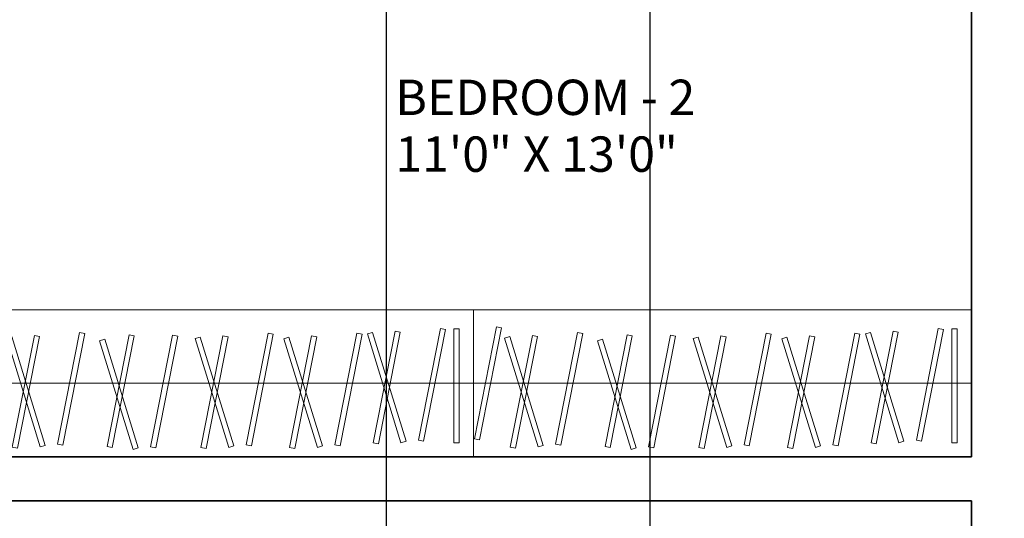
# Model space of a CAD drawing. Units: inches. Extents: x -61 to 1599, y -1316 to 257.
# Tile 145 of 204: x 406 to 540, y -16 to 52. Entities that reach past the tile are written whole.
import ezdxf

# ---------------------------------------------------------------- set-up
doc = ezdxf.new("R2010")
doc.units = ezdxf.units.IN
doc.header["$MEASUREMENT"] = 0
for name, color, linetype, lineweight in [('A-ANNO-DIMS', 2, 'Continuous', 18), ('A-AREA-IDEN', 1, 'Continuous', 18), ('A-FLOR-CASE', 8, 'Continuous', 18), ('WALLS', 4, 'Continuous', 35)]:
    doc.layers.add(name, color=color, linetype=linetype, lineweight=lineweight)
doc.styles.get("Standard").update_dxf_attribs({"font": 'arial.ttf'})
doc.dimstyles.get("Standard").update_dxf_attribs({"dimtxt": 0.18, "dimasz": 0.18, "dimexe": 0.18, "dimexo": 0.0625, "dimgap": 0.09, "dimtad": 0, "dimtih": 1, "dimtoh": 1, "dimdec": 0, "dimzin": 0, "dimdsep": 46, "dimlunit": 3, "dimtxsty": 'Standard', "dimcen": 0.09, "dimadec": 0, "dimazin": 0, "dimtfac": 1, "dimtdec": 0, "dimtofl": 0, "dimtmove": 0, "dimatfit": 3, "dimfxl": 1, "dimtolj": 1, "dimtzin": 0, "dimarcsym": 0})

# ---------------------------------------------------------------- blocks, each defined once
blk = doc.blocks.new('WARDROBE-HANGING')
blk.add_line((10.05, 0), (10.05, 68))
for points in [[(20.09, 0), (0, 0), (0, 68), (20.09, 68)], [(2.48, 67.85), (17.75, 64.85), (17.61, 64.14), (2.34, 67.15)], [(1.35, 59.16), (16.22, 63.73), (16.43, 63.04), (1.56, 58.47)], [(1.32, 62.96), (16.59, 59.95), (16.45, 59.25), (1.19, 62.25)], [(1.71, 56.78), (16.98, 53.78), (16.84, 53.07), (1.57, 56.08)], [(1, 46.47), (15.87, 51.04), (16.08, 50.35), (1.21, 45.78)], [(1.39, 50.01), (16.66, 47.01), (16.52, 46.3), (1.26, 49.31)], [(1.36, 44.09), (16.63, 41.09), (16.49, 40.38), (1.23, 43.38)], [(1.28, 33.41), (16.16, 37.98), (16.37, 37.29), (1.49, 32.72)], [(1.26, 37.2), (16.53, 34.2), (16.39, 33.49), (1.12, 36.5)], [(1.65, 31.03), (16.92, 28.03), (16.78, 27.32), (1.51, 30.32)], [(1.28, 21.3), (16.15, 25.87), (16.36, 25.18), (1.49, 20.61)], [(1.26, 25.09), (16.53, 22.09), (16.39, 21.38), (1.12, 24.39)], [(1.65, 18.92), (16.91, 15.92), (16.78, 15.21), (1.51, 18.21)], [(1.91, 13.69), (17.17, 10.68), (17.04, 9.98), (1.77, 12.98)], [(1.93, 9.89), (16.8, 14.46), (17.01, 13.77), (2.14, 9.2)], [(2.29, 7.51), (17.56, 4.51), (17.42, 3.8), (2.16, 6.81)], [(17.49, 1.96), (1.93, 1.96), (1.93, 2.68), (17.49, 2.68)]]:
    blk.add_lwpolyline(points, close=True)
blk = doc.blocks.new('*D703')
at = {"layer": 'A-ANNO-DIMS', "color": 0, "lineweight": -2, "transparency": 16777216}
for p, q in [((372.32, -616.88), (372.32, 257.46)), ((372.5, 257.28), (413.7, 257.28)), ((455.65, 257.28), (414.45, 257.28)), ((455.83, -616.88), (455.83, 257.46))]:
    blk.add_line(p, q, dxfattribs=at)
at = {"layer": 'A-ANNO-DIMS', "color": 0, "transparency": 16777216}
for points in [[(372.5, 257.31), (372.5, 257.25), (372.32, 257.28)], [(455.65, 257.31), (455.65, 257.25), (455.83, 257.28)]]:
    blk.add_solid(points, dxfattribs=at)
at = {"layer": 'DEFPOINTS', "color": 0, "transparency": 16777216}
for p in [(455.83, 257.28), (372.32, -616.94), (455.83, -616.94)]:
    blk.add_point(p, dxfattribs=at)
at = {"layer": 'A-ANNO-DIMS', "color": 0, "transparency": 16777216, "insert": (414.08, 257.28), "char_height": 0.18, "attachment_point": 5}
blk.add_mtext('\\A1;83.51', dxfattribs=at)
blk = doc.blocks.new('*D704')
at = {"layer": 'A-ANNO-DIMS', "color": 0, "lineweight": -2, "transparency": 16777216}
for p, q in [((491.83, -616.88), (491.83, 257.46)), ((492.01, 257.28), (517.87, 257.28)), ((544.52, 257.28), (518.66, 257.28)), ((544.7, -616.88), (544.7, 257.46))]:
    blk.add_line(p, q, dxfattribs=at)
at = {"layer": 'A-ANNO-DIMS', "color": 0, "transparency": 16777216}
for points in [[(492.01, 257.31), (492.01, 257.25), (491.83, 257.28)], [(544.52, 257.31), (544.52, 257.25), (544.7, 257.28)]]:
    blk.add_solid(points, dxfattribs=at)
at = {"layer": 'DEFPOINTS', "color": 0, "transparency": 16777216}
for p in [(544.7, 257.28), (491.83, -616.94), (544.7, -616.94)]:
    blk.add_point(p, dxfattribs=at)
at = {"layer": 'A-ANNO-DIMS', "color": 0, "transparency": 16777216, "insert": (518.27, 257.28), "char_height": 0.18, "attachment_point": 5}
blk.add_mtext('\\A1;52.87', dxfattribs=at)

msp = doc.modelspace()

# ---------------------------------------------------------------- linework, layer by layer
at = {"layer": 'WALLS'}
for p, q in [((535.7028, 148.6771), (535.7028, -7.3229)), ((397.7028, -7.3229), (535.7028, -7.3229)), ((397.7028, -13.3229), (535.7028, -13.3229)), ((535.7028, -13.3229), (535.7028, -175.3229))]:
    msp.add_line(p, q, dxfattribs=at)

# ---------------------------------------------------------------- block references
at = {"layer": 'A-FLOR-CASE'}
for p, rotation in [((467.7029, -7.3231), 90.00000000000017), ((535.7029, -7.3231), 90.00000000000007)]:
    msp.add_blockref('WARDROBE-HANGING', p, dxfattribs=dict(at, rotation=rotation))

# ---------------------------------------------------------------- texts
at = {"layer": 'A-AREA-IDEN'}
for s, p in [('BEDROOM - 2', (457.0332, 39.4006)), ('11\'0" X 13\'0"', (457.0332, 31.6383))]:
    msp.add_text(s, height=4.832098, dxfattribs=at).set_placement(p)

# ---------------------------------------------------------------- dimensions: what is measured, and where the dimension line sits
at = {"layer": 'A-ANNO-DIMS'}
for base, p1, p2, picture, middle in [((455.8327, 257.2771), (372.3201, -616.9446), (455.8327, -616.9446), '*D703', (414.0764, 257.2771)), ((544.7028, 257.2771), (491.8327, -616.9446), (544.7028, -616.9446), '*D704', (518.2677, 257.2771))]:
    dim = msp.add_linear_dim(base=base, p1=p1, p2=p2, dimstyle='Standard', override={"dimdec": 2, "dimlfac": 1, "dimrnd": 0, "dimzin": 0, "dimdsep": 46, "dimlunit": 2}, dxfattribs=at)
    dim.commit()
    dim.dimension.update_dxf_attribs({"geometry": picture, "text_midpoint": middle})

doc.saveas('drawing.dxf')
